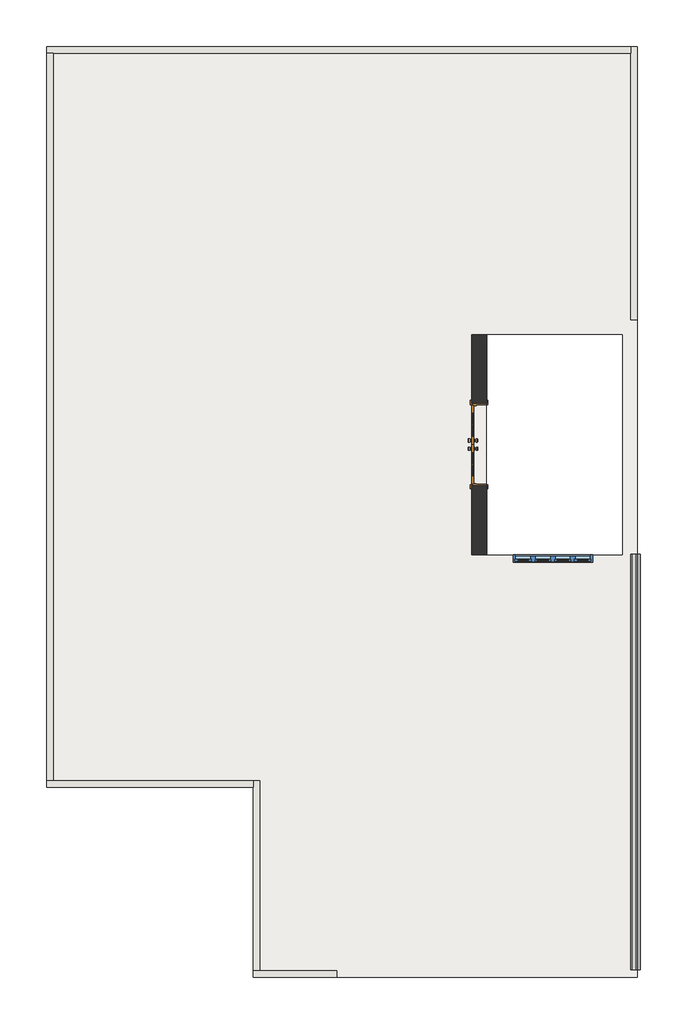
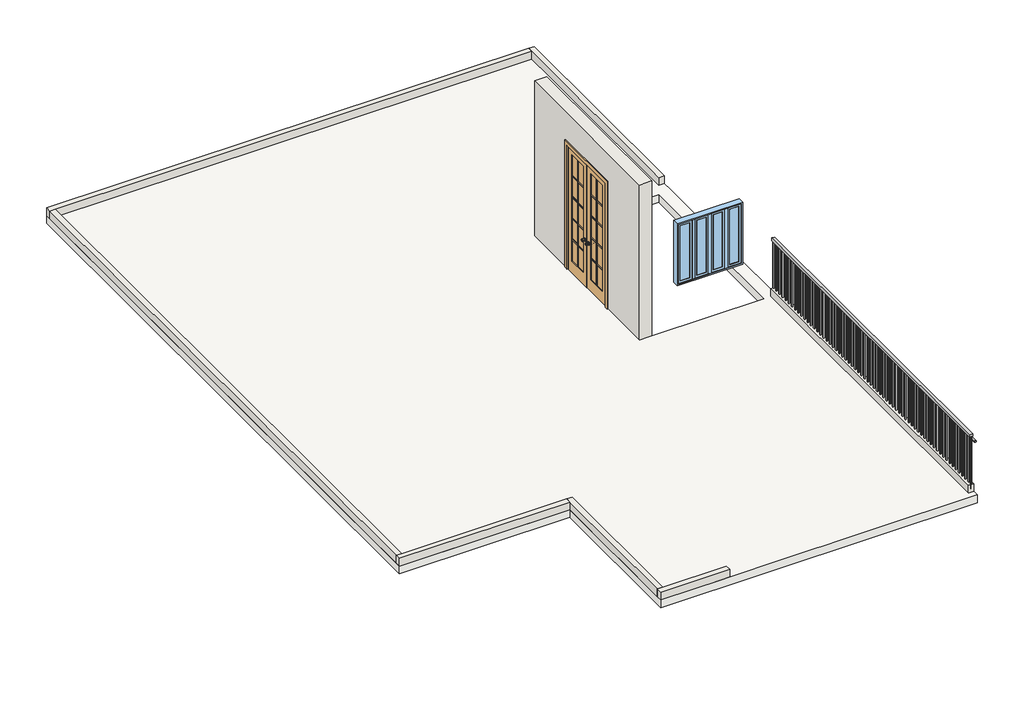
# One storey, incomplete: 8 walls, 1 door, 1 railing, 1 slab, 1 window.
"""IFC4 building model written with IfcOpenShell, lengths in millimetres."""

from ifc_helpers import new_model, si_unit, point, frame, frame_2d, origin, place, context, project, spatial, polyline, circle_curve, trimmed, segment, composite_curve, outline, extrude, faceted_brep, transform, mapped, element, save
from components import door_interior_double_full_glass_wood_4_x_8_door_7870f6d1, window_casement_multi_sash_horizontal_4_x_4_e1d7f736

model = new_model("IFC4")

# Units and contexts
model_context = context("Model", 3, world=origin())
ifc_project = project(units=[si_unit("LENGTHUNIT", "METRE", prefix="MILLI")], contexts=[model_context])

# Site, building, storey
site = spatial("IfcSite", under=ifc_project)
building = spatial("IfcBuilding", under=site)
storey = spatial("IfcBuildingStorey", under=building, Elevation=6096.0)

# Door
placement = place(None, origin())
door_interior_double_full_glass_wood_4_x_8_door_shape = door_interior_double_full_glass_wood_4_x_8_door_7870f6d1(model_context)
element("IfcDoor", 1, ObjectType="Door-Interior-Double-Full Glass-Wood : 4' X 8' DOOR", at=placement, inside=storey, context=model_context, shape_type="MappedRepresentation", body=[
    mapped(door_interior_double_full_glass_wood_4_x_8_door_shape, transform((-2038.9358498, 2841.4115866, 6096.0), x_axis=(0.0, 1.0, 0.0), y_axis=(-1.0, 0.0, 0.0), z_axis=(0.0, 0.0, 1.0))),
])

# Railing
element("IfcRailing", 2, ObjectType="Guardrail - Rectangular", at=placement, inside=storey, context=model_context, shape_type="SweptSolid", body=[
    extrude(outline(composite_curve([segment(trimmed(circle_curve(frame_2d((7067.55, 417.4391502)), 19.05), [point((7067.55, 398.3891502))], [point((7067.55, 436.4891502))], False, "CARTESIAN"), True, "CONTINUOUS"), segment(trimmed(circle_curve(frame_2d((7067.55, 417.4391502)), 19.05), [point((7067.55, 436.4891502))], [point((7067.55, 398.3891502))], False, "CARTESIAN"), True, "CONTINUOUS")], self_intersect=False)), frame((0.0, -5222.3884134, 0.0), z_axis=(0.0, 1.0, 0.0), x_axis=(0.0, 0.0, 1.0)), (0.0, 0.0, 1.0), 6377.5),
    extrude(outline(polyline([(315.8391502, 1155.1115866), (366.6391502, 1155.1115866), (366.6391502, -5222.3884134), (315.8391502, -5222.3884134), (315.8391502, 1155.1115866)])), frame((0.0, 0.0, 7188.2), z_axis=(0.0, 0.0, 1.0), x_axis=(1.0, 0.0, 0.0)), (0.0, 0.0, 1.0), 50.8),
    extrude(outline(polyline([(331.7141502, -5134.5634134), (350.7641502, -5134.5634134), (350.7641502, -5153.6134134), (331.7141502, -5153.6134134), (331.7141502, -5134.5634134)])), frame((0.0, 0.0, 6172.2), z_axis=(0.0, 0.0, 1.0), x_axis=(1.0, 0.0, 0.0)), (0.0, 0.0, 1.0), 1016.0),
    extrude(outline(polyline([(331.7141502, -5032.9634134), (350.7641502, -5032.9634134), (350.7641502, -5052.0134134), (331.7141502, -5052.0134134), (331.7141502, -5032.9634134)])), frame((0.0, 0.0, 6172.2), z_axis=(0.0, 0.0, 1.0), x_axis=(1.0, 0.0, 0.0)), (0.0, 0.0, 1.0), 1016.0),
    extrude(outline(polyline([(331.7141502, -4931.3634134), (350.7641502, -4931.3634134), (350.7641502, -4950.4134134), (331.7141502, -4950.4134134), (331.7141502, -4931.3634134)])), frame((0.0, 0.0, 6172.2), z_axis=(0.0, 0.0, 1.0), x_axis=(1.0, 0.0, 0.0)), (0.0, 0.0, 1.0), 1016.0),
    extrude(outline(polyline([(331.7141502, -4829.7634134), (350.7641502, -4829.7634134), (350.7641502, -4848.8134134), (331.7141502, -4848.8134134), (331.7141502, -4829.7634134)])), frame((0.0, 0.0, 6172.2), z_axis=(0.0, 0.0, 1.0), x_axis=(1.0, 0.0, 0.0)), (0.0, 0.0, 1.0), 1016.0),
    extrude(outline(polyline([(331.7141502, -4728.1634134), (350.7641502, -4728.1634134), (350.7641502, -4747.2134134), (331.7141502, -4747.2134134), (331.7141502, -4728.1634134)])), frame((0.0, 0.0, 6172.2), z_axis=(0.0, 0.0, 1.0), x_axis=(1.0, 0.0, 0.0)), (0.0, 0.0, 1.0), 1016.0),
    extrude(outline(polyline([(331.7141502, -4626.5634134), (350.7641502, -4626.5634134), (350.7641502, -4645.6134134), (331.7141502, -4645.6134134), (331.7141502, -4626.5634134)])), frame((0.0, 0.0, 6172.2), z_axis=(0.0, 0.0, 1.0), x_axis=(1.0, 0.0, 0.0)), (0.0, 0.0, 1.0), 1016.0),
    extrude(outline(polyline([(331.7141502, -4524.9634134), (350.7641502, -4524.9634134), (350.7641502, -4544.0134134), (331.7141502, -4544.0134134), (331.7141502, -4524.9634134)])), frame((0.0, 0.0, 6172.2), z_axis=(0.0, 0.0, 1.0), x_axis=(1.0, 0.0, 0.0)), (0.0, 0.0, 1.0), 1016.0),
    extrude(outline(polyline([(331.7141502, -4423.3634134), (350.7641502, -4423.3634134), (350.7641502, -4442.4134134), (331.7141502, -4442.4134134), (331.7141502, -4423.3634134)])), frame((0.0, 0.0, 6172.2), z_axis=(0.0, 0.0, 1.0), x_axis=(1.0, 0.0, 0.0)), (0.0, 0.0, 1.0), 1016.0),
    extrude(outline(polyline([(331.7141502, -4321.7634134), (350.7641502, -4321.7634134), (350.7641502, -4340.8134134), (331.7141502, -4340.8134134), (331.7141502, -4321.7634134)])), frame((0.0, 0.0, 6172.2), z_axis=(0.0, 0.0, 1.0), x_axis=(1.0, 0.0, 0.0)), (0.0, 0.0, 1.0), 1016.0),
    extrude(outline(polyline([(331.7141502, -4220.1634134), (350.7641502, -4220.1634134), (350.7641502, -4239.2134134), (331.7141502, -4239.2134134), (331.7141502, -4220.1634134)])), frame((0.0, 0.0, 6172.2), z_axis=(0.0, 0.0, 1.0), x_axis=(1.0, 0.0, 0.0)), (0.0, 0.0, 1.0), 1016.0),
    extrude(outline(polyline([(331.7141502, -4118.5634134), (350.7641502, -4118.5634134), (350.7641502, -4137.6134134), (331.7141502, -4137.6134134), (331.7141502, -4118.5634134)])), frame((0.0, 0.0, 6172.2), z_axis=(0.0, 0.0, 1.0), x_axis=(1.0, 0.0, 0.0)), (0.0, 0.0, 1.0), 1016.0),
    extrude(outline(polyline([(331.7141502, -4016.9634134), (350.7641502, -4016.9634134), (350.7641502, -4036.0134134), (331.7141502, -4036.0134134), (331.7141502, -4016.9634134)])), frame((0.0, 0.0, 6172.2), z_axis=(0.0, 0.0, 1.0), x_axis=(1.0, 0.0, 0.0)), (0.0, 0.0, 1.0), 1016.0),
    extrude(outline(polyline([(331.7141502, -3915.3634134), (350.7641502, -3915.3634134), (350.7641502, -3934.4134134), (331.7141502, -3934.4134134), (331.7141502, -3915.3634134)])), frame((0.0, 0.0, 6172.2), z_axis=(0.0, 0.0, 1.0), x_axis=(1.0, 0.0, 0.0)), (0.0, 0.0, 1.0), 1016.0),
    extrude(outline(polyline([(331.7141502, -3813.7634134), (350.7641502, -3813.7634134), (350.7641502, -3832.8134134), (331.7141502, -3832.8134134), (331.7141502, -3813.7634134)])), frame((0.0, 0.0, 6172.2), z_axis=(0.0, 0.0, 1.0), x_axis=(1.0, 0.0, 0.0)), (0.0, 0.0, 1.0), 1016.0),
    extrude(outline(polyline([(331.7141502, -3712.1634134), (350.7641502, -3712.1634134), (350.7641502, -3731.2134134), (331.7141502, -3731.2134134), (331.7141502, -3712.1634134)])), frame((0.0, 0.0, 6172.2), z_axis=(0.0, 0.0, 1.0), x_axis=(1.0, 0.0, 0.0)), (0.0, 0.0, 1.0), 1016.0),
    extrude(outline(polyline([(331.7141502, -3610.5634134), (350.7641502, -3610.5634134), (350.7641502, -3629.6134134), (331.7141502, -3629.6134134), (331.7141502, -3610.5634134)])), frame((0.0, 0.0, 6172.2), z_axis=(0.0, 0.0, 1.0), x_axis=(1.0, 0.0, 0.0)), (0.0, 0.0, 1.0), 1016.0),
    extrude(outline(polyline([(331.7141502, -3508.9634134), (350.7641502, -3508.9634134), (350.7641502, -3528.0134134), (331.7141502, -3528.0134134), (331.7141502, -3508.9634134)])), frame((0.0, 0.0, 6172.2), z_axis=(0.0, 0.0, 1.0), x_axis=(1.0, 0.0, 0.0)), (0.0, 0.0, 1.0), 1016.0),
    extrude(outline(polyline([(331.7141502, -3407.3634134), (350.7641502, -3407.3634134), (350.7641502, -3426.4134134), (331.7141502, -3426.4134134), (331.7141502, -3407.3634134)])), frame((0.0, 0.0, 6172.2), z_axis=(0.0, 0.0, 1.0), x_axis=(1.0, 0.0, 0.0)), (0.0, 0.0, 1.0), 1016.0),
    extrude(outline(polyline([(331.7141502, -3305.7634134), (350.7641502, -3305.7634134), (350.7641502, -3324.8134134), (331.7141502, -3324.8134134), (331.7141502, -3305.7634134)])), frame((0.0, 0.0, 6172.2), z_axis=(0.0, 0.0, 1.0), x_axis=(1.0, 0.0, 0.0)), (0.0, 0.0, 1.0), 1016.0),
    extrude(outline(polyline([(331.7141502, -3204.1634134), (350.7641502, -3204.1634134), (350.7641502, -3223.2134134), (331.7141502, -3223.2134134), (331.7141502, -3204.1634134)])), frame((0.0, 0.0, 6172.2), z_axis=(0.0, 0.0, 1.0), x_axis=(1.0, 0.0, 0.0)), (0.0, 0.0, 1.0), 1016.0),
    extrude(outline(polyline([(331.7141502, -3102.5634134), (350.7641502, -3102.5634134), (350.7641502, -3121.6134134), (331.7141502, -3121.6134134), (331.7141502, -3102.5634134)])), frame((0.0, 0.0, 6172.2), z_axis=(0.0, 0.0, 1.0), x_axis=(1.0, 0.0, 0.0)), (0.0, 0.0, 1.0), 1016.0),
    extrude(outline(polyline([(331.7141502, -3000.9634134), (350.7641502, -3000.9634134), (350.7641502, -3020.0134134), (331.7141502, -3020.0134134), (331.7141502, -3000.9634134)])), frame((0.0, 0.0, 6172.2), z_axis=(0.0, 0.0, 1.0), x_axis=(1.0, 0.0, 0.0)), (0.0, 0.0, 1.0), 1016.0),
    extrude(outline(polyline([(331.7141502, -2899.3634134), (350.7641502, -2899.3634134), (350.7641502, -2918.4134134), (331.7141502, -2918.4134134), (331.7141502, -2899.3634134)])), frame((0.0, 0.0, 6172.2), z_axis=(0.0, 0.0, 1.0), x_axis=(1.0, 0.0, 0.0)), (0.0, 0.0, 1.0), 1016.0),
    extrude(outline(polyline([(331.7141502, -2797.7634134), (350.7641502, -2797.7634134), (350.7641502, -2816.8134134), (331.7141502, -2816.8134134), (331.7141502, -2797.7634134)])), frame((0.0, 0.0, 6172.2), z_axis=(0.0, 0.0, 1.0), x_axis=(1.0, 0.0, 0.0)), (0.0, 0.0, 1.0), 1016.0),
    extrude(outline(polyline([(331.7141502, -2696.1634134), (350.7641502, -2696.1634134), (350.7641502, -2715.2134134), (331.7141502, -2715.2134134), (331.7141502, -2696.1634134)])), frame((0.0, 0.0, 6172.2), z_axis=(0.0, 0.0, 1.0), x_axis=(1.0, 0.0, 0.0)), (0.0, 0.0, 1.0), 1016.0),
    extrude(outline(polyline([(331.7141502, -2594.5634134), (350.7641502, -2594.5634134), (350.7641502, -2613.6134134), (331.7141502, -2613.6134134), (331.7141502, -2594.5634134)])), frame((0.0, 0.0, 6172.2), z_axis=(0.0, 0.0, 1.0), x_axis=(1.0, 0.0, 0.0)), (0.0, 0.0, 1.0), 1016.0),
    extrude(outline(polyline([(331.7141502, -2492.9634134), (350.7641502, -2492.9634134), (350.7641502, -2512.0134134), (331.7141502, -2512.0134134), (331.7141502, -2492.9634134)])), frame((0.0, 0.0, 6172.2), z_axis=(0.0, 0.0, 1.0), x_axis=(1.0, 0.0, 0.0)), (0.0, 0.0, 1.0), 1016.0),
    extrude(outline(polyline([(331.7141502, -2391.3634134), (350.7641502, -2391.3634134), (350.7641502, -2410.4134134), (331.7141502, -2410.4134134), (331.7141502, -2391.3634134)])), frame((0.0, 0.0, 6172.2), z_axis=(0.0, 0.0, 1.0), x_axis=(1.0, 0.0, 0.0)), (0.0, 0.0, 1.0), 1016.0),
    extrude(outline(polyline([(331.7141502, -2289.7634134), (350.7641502, -2289.7634134), (350.7641502, -2308.8134134), (331.7141502, -2308.8134134), (331.7141502, -2289.7634134)])), frame((0.0, 0.0, 6172.2), z_axis=(0.0, 0.0, 1.0), x_axis=(1.0, 0.0, 0.0)), (0.0, 0.0, 1.0), 1016.0),
    extrude(outline(polyline([(331.7141502, -2188.1634134), (350.7641502, -2188.1634134), (350.7641502, -2207.2134134), (331.7141502, -2207.2134134), (331.7141502, -2188.1634134)])), frame((0.0, 0.0, 6172.2), z_axis=(0.0, 0.0, 1.0), x_axis=(1.0, 0.0, 0.0)), (0.0, 0.0, 1.0), 1016.0),
    extrude(outline(polyline([(331.7141502, -2086.5634134), (350.7641502, -2086.5634134), (350.7641502, -2105.6134134), (331.7141502, -2105.6134134), (331.7141502, -2086.5634134)])), frame((0.0, 0.0, 6172.2), z_axis=(0.0, 0.0, 1.0), x_axis=(1.0, 0.0, 0.0)), (0.0, 0.0, 1.0), 1016.0),
    extrude(outline(polyline([(331.7141502, -1984.9634134), (350.7641502, -1984.9634134), (350.7641502, -2004.0134134), (331.7141502, -2004.0134134), (331.7141502, -1984.9634134)])), frame((0.0, 0.0, 6172.2), z_axis=(0.0, 0.0, 1.0), x_axis=(1.0, 0.0, 0.0)), (0.0, 0.0, 1.0), 1016.0),
    extrude(outline(polyline([(331.7141502, -1883.3634134), (350.7641502, -1883.3634134), (350.7641502, -1902.4134134), (331.7141502, -1902.4134134), (331.7141502, -1883.3634134)])), frame((0.0, 0.0, 6172.2), z_axis=(0.0, 0.0, 1.0), x_axis=(1.0, 0.0, 0.0)), (0.0, 0.0, 1.0), 1016.0),
    extrude(outline(polyline([(331.7141502, -1781.7634134), (350.7641502, -1781.7634134), (350.7641502, -1800.8134134), (331.7141502, -1800.8134134), (331.7141502, -1781.7634134)])), frame((0.0, 0.0, 6172.2), z_axis=(0.0, 0.0, 1.0), x_axis=(1.0, 0.0, 0.0)), (0.0, 0.0, 1.0), 1016.0),
    extrude(outline(polyline([(331.7141502, -1680.1634134), (350.7641502, -1680.1634134), (350.7641502, -1699.2134134), (331.7141502, -1699.2134134), (331.7141502, -1680.1634134)])), frame((0.0, 0.0, 6172.2), z_axis=(0.0, 0.0, 1.0), x_axis=(1.0, 0.0, 0.0)), (0.0, 0.0, 1.0), 1016.0),
    extrude(outline(polyline([(331.7141502, -1578.5634134), (350.7641502, -1578.5634134), (350.7641502, -1597.6134134), (331.7141502, -1597.6134134), (331.7141502, -1578.5634134)])), frame((0.0, 0.0, 6172.2), z_axis=(0.0, 0.0, 1.0), x_axis=(1.0, 0.0, 0.0)), (0.0, 0.0, 1.0), 1016.0),
    extrude(outline(polyline([(331.7141502, -1476.9634134), (350.7641502, -1476.9634134), (350.7641502, -1496.0134134), (331.7141502, -1496.0134134), (331.7141502, -1476.9634134)])), frame((0.0, 0.0, 6172.2), z_axis=(0.0, 0.0, 1.0), x_axis=(1.0, 0.0, 0.0)), (0.0, 0.0, 1.0), 1016.0),
    extrude(outline(polyline([(331.7141502, -1375.3634134), (350.7641502, -1375.3634134), (350.7641502, -1394.4134134), (331.7141502, -1394.4134134), (331.7141502, -1375.3634134)])), frame((0.0, 0.0, 6172.2), z_axis=(0.0, 0.0, 1.0), x_axis=(1.0, 0.0, 0.0)), (0.0, 0.0, 1.0), 1016.0),
    extrude(outline(polyline([(331.7141502, -1273.7634134), (350.7641502, -1273.7634134), (350.7641502, -1292.8134134), (331.7141502, -1292.8134134), (331.7141502, -1273.7634134)])), frame((0.0, 0.0, 6172.2), z_axis=(0.0, 0.0, 1.0), x_axis=(1.0, 0.0, 0.0)), (0.0, 0.0, 1.0), 1016.0),
    extrude(outline(polyline([(331.7141502, -1172.1634134), (350.7641502, -1172.1634134), (350.7641502, -1191.2134134), (331.7141502, -1191.2134134), (331.7141502, -1172.1634134)])), frame((0.0, 0.0, 6172.2), z_axis=(0.0, 0.0, 1.0), x_axis=(1.0, 0.0, 0.0)), (0.0, 0.0, 1.0), 1016.0),
    extrude(outline(polyline([(331.7141502, -1070.5634134), (350.7641502, -1070.5634134), (350.7641502, -1089.6134134), (331.7141502, -1089.6134134), (331.7141502, -1070.5634134)])), frame((0.0, 0.0, 6172.2), z_axis=(0.0, 0.0, 1.0), x_axis=(1.0, 0.0, 0.0)), (0.0, 0.0, 1.0), 1016.0),
    extrude(outline(polyline([(331.7141502, -968.9634134), (350.7641502, -968.9634134), (350.7641502, -988.0134134), (331.7141502, -988.0134134), (331.7141502, -968.9634134)])), frame((0.0, 0.0, 6172.2), z_axis=(0.0, 0.0, 1.0), x_axis=(1.0, 0.0, 0.0)), (0.0, 0.0, 1.0), 1016.0),
    extrude(outline(polyline([(331.7141502, -867.3634134), (350.7641502, -867.3634134), (350.7641502, -886.4134134), (331.7141502, -886.4134134), (331.7141502, -867.3634134)])), frame((0.0, 0.0, 6172.2), z_axis=(0.0, 0.0, 1.0), x_axis=(1.0, 0.0, 0.0)), (0.0, 0.0, 1.0), 1016.0),
    extrude(outline(polyline([(331.7141502, -765.7634134), (350.7641502, -765.7634134), (350.7641502, -784.8134134), (331.7141502, -784.8134134), (331.7141502, -765.7634134)])), frame((0.0, 0.0, 6172.2), z_axis=(0.0, 0.0, 1.0), x_axis=(1.0, 0.0, 0.0)), (0.0, 0.0, 1.0), 1016.0),
    extrude(outline(polyline([(331.7141502, -664.1634134), (350.7641502, -664.1634134), (350.7641502, -683.2134134), (331.7141502, -683.2134134), (331.7141502, -664.1634134)])), frame((0.0, 0.0, 6172.2), z_axis=(0.0, 0.0, 1.0), x_axis=(1.0, 0.0, 0.0)), (0.0, 0.0, 1.0), 1016.0),
    extrude(outline(polyline([(331.7141502, -562.5634134), (350.7641502, -562.5634134), (350.7641502, -581.6134134), (331.7141502, -581.6134134), (331.7141502, -562.5634134)])), frame((0.0, 0.0, 6172.2), z_axis=(0.0, 0.0, 1.0), x_axis=(1.0, 0.0, 0.0)), (0.0, 0.0, 1.0), 1016.0),
    extrude(outline(polyline([(331.7141502, -460.9634134), (350.7641502, -460.9634134), (350.7641502, -480.0134134), (331.7141502, -480.0134134), (331.7141502, -460.9634134)])), frame((0.0, 0.0, 6172.2), z_axis=(0.0, 0.0, 1.0), x_axis=(1.0, 0.0, 0.0)), (0.0, 0.0, 1.0), 1016.0),
    extrude(outline(polyline([(331.7141502, -359.3634134), (350.7641502, -359.3634134), (350.7641502, -378.4134134), (331.7141502, -378.4134134), (331.7141502, -359.3634134)])), frame((0.0, 0.0, 6172.2), z_axis=(0.0, 0.0, 1.0), x_axis=(1.0, 0.0, 0.0)), (0.0, 0.0, 1.0), 1016.0),
    extrude(outline(polyline([(331.7141502, -257.7634134), (350.7641502, -257.7634134), (350.7641502, -276.8134134), (331.7141502, -276.8134134), (331.7141502, -257.7634134)])), frame((0.0, 0.0, 6172.2), z_axis=(0.0, 0.0, 1.0), x_axis=(1.0, 0.0, 0.0)), (0.0, 0.0, 1.0), 1016.0),
    extrude(outline(polyline([(331.7141502, -156.1634134), (350.7641502, -156.1634134), (350.7641502, -175.2134134), (331.7141502, -175.2134134), (331.7141502, -156.1634134)])), frame((0.0, 0.0, 6172.2), z_axis=(0.0, 0.0, 1.0), x_axis=(1.0, 0.0, 0.0)), (0.0, 0.0, 1.0), 1016.0),
    extrude(outline(polyline([(331.7141502, -54.5634134), (350.7641502, -54.5634134), (350.7641502, -73.6134134), (331.7141502, -73.6134134), (331.7141502, -54.5634134)])), frame((0.0, 0.0, 6172.2), z_axis=(0.0, 0.0, 1.0), x_axis=(1.0, 0.0, 0.0)), (0.0, 0.0, 1.0), 1016.0),
    extrude(outline(polyline([(331.7141502, 47.0365866), (350.7641502, 47.0365866), (350.7641502, 27.9865866), (331.7141502, 27.9865866), (331.7141502, 47.0365866)])), frame((0.0, 0.0, 6172.2), z_axis=(0.0, 0.0, 1.0), x_axis=(1.0, 0.0, 0.0)), (0.0, 0.0, 1.0), 1016.0),
    extrude(outline(polyline([(331.7141502, 148.6365866), (350.7641502, 148.6365866), (350.7641502, 129.5865866), (331.7141502, 129.5865866), (331.7141502, 148.6365866)])), frame((0.0, 0.0, 6172.2), z_axis=(0.0, 0.0, 1.0), x_axis=(1.0, 0.0, 0.0)), (0.0, 0.0, 1.0), 1016.0),
    extrude(outline(polyline([(331.7141502, 250.2365866), (350.7641502, 250.2365866), (350.7641502, 231.1865866), (331.7141502, 231.1865866), (331.7141502, 250.2365866)])), frame((0.0, 0.0, 6172.2), z_axis=(0.0, 0.0, 1.0), x_axis=(1.0, 0.0, 0.0)), (0.0, 0.0, 1.0), 1016.0),
    extrude(outline(polyline([(331.7141502, 351.8365866), (350.7641502, 351.8365866), (350.7641502, 332.7865866), (331.7141502, 332.7865866), (331.7141502, 351.8365866)])), frame((0.0, 0.0, 6172.2), z_axis=(0.0, 0.0, 1.0), x_axis=(1.0, 0.0, 0.0)), (0.0, 0.0, 1.0), 1016.0),
    extrude(outline(polyline([(331.7141502, 453.4365866), (350.7641502, 453.4365866), (350.7641502, 434.3865866), (331.7141502, 434.3865866), (331.7141502, 453.4365866)])), frame((0.0, 0.0, 6172.2), z_axis=(0.0, 0.0, 1.0), x_axis=(1.0, 0.0, 0.0)), (0.0, 0.0, 1.0), 1016.0),
    extrude(outline(polyline([(331.7141502, 555.0365866), (350.7641502, 555.0365866), (350.7641502, 535.9865866), (331.7141502, 535.9865866), (331.7141502, 555.0365866)])), frame((0.0, 0.0, 6172.2), z_axis=(0.0, 0.0, 1.0), x_axis=(1.0, 0.0, 0.0)), (0.0, 0.0, 1.0), 1016.0),
    extrude(outline(polyline([(331.7141502, 656.6365866), (350.7641502, 656.6365866), (350.7641502, 637.5865866), (331.7141502, 637.5865866), (331.7141502, 656.6365866)])), frame((0.0, 0.0, 6172.2), z_axis=(0.0, 0.0, 1.0), x_axis=(1.0, 0.0, 0.0)), (0.0, 0.0, 1.0), 1016.0),
    extrude(outline(polyline([(331.7141502, 758.2365866), (350.7641502, 758.2365866), (350.7641502, 739.1865866), (331.7141502, 739.1865866), (331.7141502, 758.2365866)])), frame((0.0, 0.0, 6172.2), z_axis=(0.0, 0.0, 1.0), x_axis=(1.0, 0.0, 0.0)), (0.0, 0.0, 1.0), 1016.0),
    extrude(outline(polyline([(331.7141502, 859.8365866), (350.7641502, 859.8365866), (350.7641502, 840.7865866), (331.7141502, 840.7865866), (331.7141502, 859.8365866)])), frame((0.0, 0.0, 6172.2), z_axis=(0.0, 0.0, 1.0), x_axis=(1.0, 0.0, 0.0)), (0.0, 0.0, 1.0), 1016.0),
    extrude(outline(polyline([(331.7141502, 961.4365866), (350.7641502, 961.4365866), (350.7641502, 942.3865866), (331.7141502, 942.3865866), (331.7141502, 961.4365866)])), frame((0.0, 0.0, 6172.2), z_axis=(0.0, 0.0, 1.0), x_axis=(1.0, 0.0, 0.0)), (0.0, 0.0, 1.0), 1016.0),
    extrude(outline(polyline([(331.7141502, 1063.0365866), (350.7641502, 1063.0365866), (350.7641502, 1043.9865866), (331.7141502, 1043.9865866), (331.7141502, 1063.0365866)])), frame((0.0, 0.0, 6172.2), z_axis=(0.0, 0.0, 1.0), x_axis=(1.0, 0.0, 0.0)), (0.0, 0.0, 1.0), 1016.0),
    extrude(outline(polyline([(331.7141502, -5203.3384134), (350.7641502, -5203.3384134), (350.7641502, -5222.3884134), (331.7141502, -5222.3884134), (331.7141502, -5203.3384134)])), frame((0.0, 0.0, 6172.2), z_axis=(0.0, 0.0, 1.0), x_axis=(1.0, 0.0, 0.0)), (0.0, 0.0, 1.0), 1016.0),
    extrude(outline(polyline([(331.7141502, 1155.1115866), (350.7641502, 1155.1115866), (350.7641502, 1136.0615866), (331.7141502, 1136.0615866), (331.7141502, 1155.1115866)])), frame((0.0, 0.0, 6172.2), z_axis=(0.0, 0.0, 1.0), x_axis=(1.0, 0.0, 0.0)), (0.0, 0.0, 1.0), 1016.0),
])

# Slab
element("IfcSlab", 3, ObjectType="6\" FLOOR", at=placement, inside=storey, context=model_context, shape_type="SweptSolid", body=[
    extrude(outline(polyline([(-8677.1608498, 8952.9115866), (392.0391502, 8952.9115866), (392.0391502, -5337.3884134), (-5503.5608498, -5337.3884134), (-5503.5608498, -2415.6884134), (-8677.1608498, -2415.6884134), (-8677.1608498, 8952.9115866)]), holes=[polyline([(162.0391502, 1152.3115866), (162.0391502, 4530.5115866), (-1920.7608498, 4530.5115866), (-1920.7608498, 1152.3115866), (162.0391502, 1152.3115866)])]), frame((0.0, 0.0, 5943.6), z_axis=(0.0, 0.0, 1.0), x_axis=(1.0, 0.0, 0.0)), (0.0, 0.0, 1.0), 152.4),
])

# Walls
element("IfcWall", 4, ObjectType="4\" wall", at=placement, inside=storey, context=model_context, shape_type="Brep", body=[
    faceted_brep([(-4220.1608498, -5236.4884134, 6096.0), (-5401.9608498, -5236.4884134, 6096.0), (-5503.5608498, -5236.4884134, 6096.0), (-5503.5608498, -5236.4884134, 6248.4), (-5401.9608498, -5236.4884134, 6248.4), (-4220.1608498, -5236.4884134, 6248.4), (-4220.1608498, -5338.0884134, 6096.0), (-4220.1608498, -5338.0884134, 6248.4), (-5503.5608498, -5338.0884134, 6248.4), (-5503.5608498, -5338.0884134, 6096.0), (-4335.1608498, -5338.0884134, 6096.0)], [[[0, 1, 2, 3, 4, 5]], [[6, 7, 8, 9, 10]], [[2, 1, 0, 6, 10, 9]], [[5, 4, 3, 8, 7]], [[0, 5, 7, 6]], [[3, 2, 9, 8]]]),
])
element("IfcWall", 5, ObjectType="4\" wall", at=placement, inside=storey, context=model_context, shape_type="Brep", body=[
    faceted_brep([(-5401.9608498, -5236.4884134, 6096.0), (-5401.9608498, -2315.4884134, 6096.0), (-5401.9608498, -2315.4884134, 6248.4), (-5401.9608498, -5236.4884134, 6248.4), (-5503.5608498, -5236.4884134, 6096.0), (-5503.5608498, -5236.4884134, 6248.4), (-5503.5608498, -2417.0884134, 6248.4), (-5503.5608498, -2315.4884134, 6248.4), (-5503.5608498, -2315.4884134, 6096.0), (-5503.5608498, -2417.0884134, 6096.0)], [[[0, 1, 2, 3]], [[4, 5, 6, 7, 8, 9]], [[1, 0, 4, 9, 8]], [[3, 2, 7, 6, 5]], [[0, 3, 5, 4]], [[2, 1, 8, 7]]]),
])
element("IfcWall", 6, ObjectType="4\" wall", at=placement, inside=storey, context=model_context, shape_type="Brep", body=[
    faceted_brep([(-5503.5608498, -2315.4884134, 6096.0), (-8575.5608498, -2315.4884134, 6096.0), (-8677.1608498, -2315.4884134, 6096.0), (-8677.1608498, -2315.4884134, 6248.4), (-8575.5608498, -2315.4884134, 6248.4), (-5503.5608498, -2315.4884134, 6248.4), (-5503.5608498, -2417.0884134, 6096.0), (-5503.5608498, -2417.0884134, 6248.4), (-8677.1608498, -2417.0884134, 6248.4), (-8677.1608498, -2417.0884134, 6096.0)], [[[0, 1, 2, 3, 4, 5]], [[6, 7, 8, 9]], [[2, 1, 0, 6, 9]], [[5, 4, 3, 8, 7]], [[0, 5, 7, 6]], [[3, 2, 9, 8]]]),
])
element("IfcWall", 7, ObjectType="4\" wall", at=placement, inside=storey, context=model_context, shape_type="Brep", body=[
    faceted_brep([(392.0391502, 4760.5115866, 6096.0), (392.0391502, 8952.9115866, 6096.0), (392.0391502, 8952.9115866, 6248.4), (392.0391502, 4760.5115866, 6248.4), (290.4391502, 4760.5115866, 6096.0), (290.4391502, 4760.5115866, 6248.4), (290.4391502, 8851.3115866, 6248.4), (290.4391502, 8952.9115866, 6248.4), (290.4391502, 8952.9115866, 6096.0), (290.4391502, 8851.3115866, 6096.0)], [[[0, 1, 2, 3]], [[4, 5, 6, 7, 8, 9]], [[1, 0, 4, 9, 8]], [[3, 2, 7, 6, 5]], [[0, 3, 5, 4]], [[2, 1, 8, 7]]]),
])
element("IfcWall", 8, ObjectType="4\" wall", at=placement, inside=storey, context=model_context, shape_type="Brep", body=[
    faceted_brep([(290.4391502, 8952.9115866, 6096.0), (-8677.1608498, 8952.9115866, 6096.0), (-8677.1608498, 8952.9115866, 6248.4), (290.4391502, 8952.9115866, 6248.4), (290.4391502, 8851.3115866, 6096.0), (290.4391502, 8851.3115866, 6248.4), (-8575.5608498, 8851.3115866, 6248.4), (-8677.1608498, 8851.3115866, 6248.4), (-8677.1608498, 8851.3115866, 6096.0), (-8575.5608498, 8851.3115866, 6096.0)], [[[0, 1, 2, 3]], [[4, 5, 6, 7, 8, 9]], [[1, 0, 4, 9, 8]], [[3, 2, 7, 6, 5]], [[0, 3, 5, 4]], [[2, 1, 8, 7]]]),
])
element("IfcWall", 9, ObjectType="4\" wall", at=placement, inside=storey, context=model_context, shape_type="SweptSolid", body=[
    extrude(outline(polyline([(-8677.1608498, -2315.4884134), (-8677.1608498, 8851.3115866), (-8575.5608498, 8851.3115866), (-8575.5608498, -2315.4884134), (-8677.1608498, -2315.4884134)])), frame((0.0, 0.0, 6096.0), z_axis=(0.0, 0.0, 1.0), x_axis=(1.0, 0.0, 0.0)), (0.0, 0.0, 1.0), 152.4),
])
element("IfcWall", 10, ObjectType="4\" wall", at=placement, inside=storey, context=model_context, shape_type="Brep", body=[
    faceted_brep([(392.0391502, -5222.3884134, 6096.0), (392.0391502, -5108.0884134, 6096.0), (392.0391502, 1155.1115866, 6096.0), (392.0391502, 1155.1115866, 6248.4), (392.0391502, -5222.3884134, 6248.4), (290.4391502, -5222.3884134, 6096.0), (290.4391502, -5222.3884134, 6248.4), (290.4391502, 1155.1115866, 6248.4), (290.4391502, 1155.1115866, 6096.0)], [[[0, 1, 2, 3, 4]], [[5, 6, 7, 8]], [[2, 1, 0, 5, 8]], [[3, 2, 8, 7]], [[4, 3, 7, 6]], [[0, 4, 6, 5]]]),
])
element("IfcWall", 11, ObjectType="9\" wall", at=placement, inside=storey, context=model_context, shape_type="Brep", body=[
    faceted_brep([(-2150.7608498, 1152.3115866, 9144.0), (-2150.7608498, 4530.5115866, 9144.0), (-2150.7608498, 4530.5115866, 6096.0), (-2150.7608498, 3476.4115866, 6096.0), (-2150.7608498, 3476.4115866, 8559.8), (-2150.7608498, 2206.4115866, 8559.8), (-2150.7608498, 2206.4115866, 6096.0), (-2150.7608498, 1152.3115866, 6096.0), (-1920.7608498, 4530.5115866, 9144.0), (-1920.7608498, 1152.3115866, 9144.0), (-1920.7608498, 1152.3115866, 6096.0), (-1920.7608498, 2206.4115866, 6096.0), (-1920.7608498, 2206.4115866, 8559.8), (-1920.7608498, 3476.4115866, 8559.8), (-1920.7608498, 3476.4115866, 6096.0), (-1920.7608498, 4530.5115866, 6096.0), (-2035.7608498, 4530.5115866, 6096.0), (-2035.7608498, 1152.3115866, 6096.0)], [[[0, 1, 2, 3, 4, 5, 6, 7]], [[8, 9, 10, 11, 12, 13, 14, 15]], [[2, 16, 15, 14, 3]], [[10, 17, 7, 6, 11]], [[1, 0, 9, 8]], [[2, 1, 8, 15, 16]], [[0, 7, 17, 10, 9]], [[13, 4, 3, 14]], [[4, 13, 12, 5]], [[5, 12, 11, 6]]]),
])

# Window
window_casement_multi_sash_horizontal_4_x_4_shape = window_casement_multi_sash_horizontal_4_x_4_e1d7f736(model_context)
element("IfcWindow", 12, ObjectType="Window-Casement-Multi-Sash-Horizontal : 4' x 4'", at=placement, inside=storey, context=model_context, shape_type="MappedRepresentation", body=[
    mapped(window_casement_multi_sash_horizontal_4_x_4_shape, transform((-904.7608498, 1095.1615866, 6096.0), x_axis=(-1.0, 0.0, 0.0), y_axis=(0.0, -1.0, 0.0), z_axis=(0.0, 0.0, 1.0))),
])

save(model, "model.ifc")

# Revit data of these elements
# Type "Door-Interior-Double-Full Glass-Wood : 4' X 8' DOOR"
#   Type Mark = "12"
#   Assembly Code = "C1020300"
#   Analytic Construction = "French door, wood frame with single glass"
#   Top Rail = 0' - 4 11/16"
#   Thickness = 0' - 1 3/8"
#   Thermal Resistance (R) = 1.0696 (h·ft²·°F)/BTU
#   Swing Angle [instance default] = 90.00°
#   Stiles = 0' - 4 3/4"
#   Rough Width = 4' - 2"
#   Rough Height = 8' - 1"
#   Panel Width = 2' - 0"
#   Height = 8' - 0"
#   Width = 4' - 0"
#   Heat Transfer Coefficient (U) = 0.9350 BTU/(h·ft²·°F)
#   Bottom Rail = 0' - 9 1/8"
#   Show Grill [instance default] = yes
#   Trim Material = Cherry
#   Panel Material = Cherry
#   Frame Material = Cherry
#   Door Handle Material = Aluminum
#   Visual Light Transmittance = 0
#   Solar Heat Gain Coefficient = 0
#   Wall Closure = (empty or 0)
#   Function = (empty or 0)
# Type "Guardrail - Rectangular"
#   Assembly Code = "C2010400"
#   built-in parameter 1008612 = 0.0416667 (stored number, unit not read)
#   built-in parameter 1008611 = 0.0416667 (stored number, unit not read)
#   built-in parameter 1008609 = 0.333333 (stored number, unit not read)
#   built-in parameter 1008604 = 0.166667 (stored number, unit not read)
#   built-in parameter 1008603 = 0.166667 (stored number, unit not read)
#   Railing Height = 3' - 6"
#   built-in parameter 1008630 = 2
#   built-in parameter 1008610 = 1
#   built-in parameter 1008618 = Baluster - Square : 3/4"
# Type "6\" FLOOR"
#   Assembly Code = "B1010"
#   Function = 0
#   Layers, outside or top first: 0' - 6" no material (function 1)
# Type "4\" wall"
#   Assembly Code = "B2010"
#   Layers, outside or top first: 0' - 4" no material (function 1)
# Type "9\" wall"
#   Assembly Code = "B2010"
#   Layers, outside or top first: 0' - 9 7/128" no material (function 1)
# Type "Window-Casement-Multi-Sash-Horizontal : 4' x 4'"
#   Type Mark = "W1"
#   Fire Rating = "0.5h"
#   Assembly Code = "B2020100"
#   Analytic Construction = "Double glazing - domestic"
#   Window Inset [instance default] = 0' - 0 5/8"
#   Wall Thickness [instance default] = 0' - 6"
#   Visual Light Transmittance = 0.81
#   Thermal Resistance (R) = 1.8146 (h·ft²·°F)/BTU
#   Solar Heat Gain Coefficient = 0.76
#   Rough Width = 4' - 0 1/2"
#   Rough Height = 4' - 0 1/2"
#   Open Window Width = 1' - 0"
#   Heat Transfer Coefficient (U) = 0.5511 BTU/(h·ft²·°F)
#   Height = 4' - 0"
#   Frame Gap 3 [instance default] = 0' - 1 83/128"
#   Frame Gap 2 [instance default] = 0' - 0 5/8"
#   Frame Gap 1 = 0' - 1 51/128"
#   Default Sill Height = 3' - 0"
#   Width = 4' - 0"
#   Frame Material = Metal - Aluminum
#   Glass Panel Material = Glass
#   Wall Closure = (empty or 0)
# Element 1 (IfcDoor, "Door-Interior-Double-Full Glass-Wood : 4' X 8' DOOR")
#   Swing Angle = 90.00°
#   Show Grill = yes
#   Phase Created = New Construction
#   Materials on its faces: "Cherry", "Aluminum", "Glass"
# Element 2 (IfcRailing, "Guardrail - Rectangular")
#   built-in parameter 1008621 = 0.25 (stored number, unit not read)
#   Phase Created = New Construction
# Element 3 (IfcSlab, "6\" FLOOR")
#   built-in parameter 1001955 = 3.14159 (stored number, unit not read)
#   Height Offset From Level = 0' - 0"
#   Phase Created = New Construction
#   Materials on its faces: "Default Floor", "white colour"
# Elements 4, 5, 6, 7, 8 (IfcWall, "4\" wall")
#   Top Offset = 0' - 0"
#   Base Offset = 0' - 0"
#   Unconnected Height = 0' - 6"
#   wall height = 0' - 6"
#   Phase Created = New Construction
#   Materials on its faces: "white colour", "Default Wall"
# Elements 9, 10 (IfcWall, "4\" wall")
#   Top Offset = 0' - 0"
#   Base Offset = 0' - 0"
#   Unconnected Height = 0' - 6"
#   wall height = 0' - 6"
#   Phase Created = New Construction
#   Materials on its faces: "Default Wall", "white colour"
# Element 11 (IfcWall, "9\" wall")
#   Top Offset = 0' - 0"
#   Base Offset = 0' - 0"
#   wall height = 10' - 0"
#   Phase Created = New Construction
#   Materials on its faces: "Default Wall", "Main wall"
# Element 12 (IfcWindow, "Window-Casement-Multi-Sash-Horizontal : 4' x 4'")
#   Mark = "14"
#   Window Inset = 0' - 0 5/8"
#   Frame Gap 3 = 0' - 1 83/128"
#   Frame Gap 2 = 0' - 0 5/8"
#   Phase Created = New Construction
#   Materials on its faces: "Metal - Aluminum", "Glass"
# Materials
#   "Cherry": class "Wood", colour RGB 226 177 128, transparency 0, Description = "Prunus Serotina", Cost = 0
#   "Aluminum": class "Metal", colour RGB 247 247 247, transparency 0, Description = "Aluminum 6061", Cost = 0
#   "Metal - Aluminum": class "Metal", colour RGB 247 247 247, transparency 0
#   "Glass": class "Glass", colour RGB 0 128 192, transparency 0.75, Description = "Soda Lime Glass", Cost = 0
#   "Default Floor": colour RGB 128 128 128, transparency 0, Cost = 0
#   "white colour": class "Generic", colour RGB 120 120 120, transparency 0, Cost = 0
#   "Default Wall": colour RGB 128 128 128, transparency 0, Cost = 0
#   "Main wall": class "Generic", colour RGB 120 120 120, transparency 0, Cost = 0
